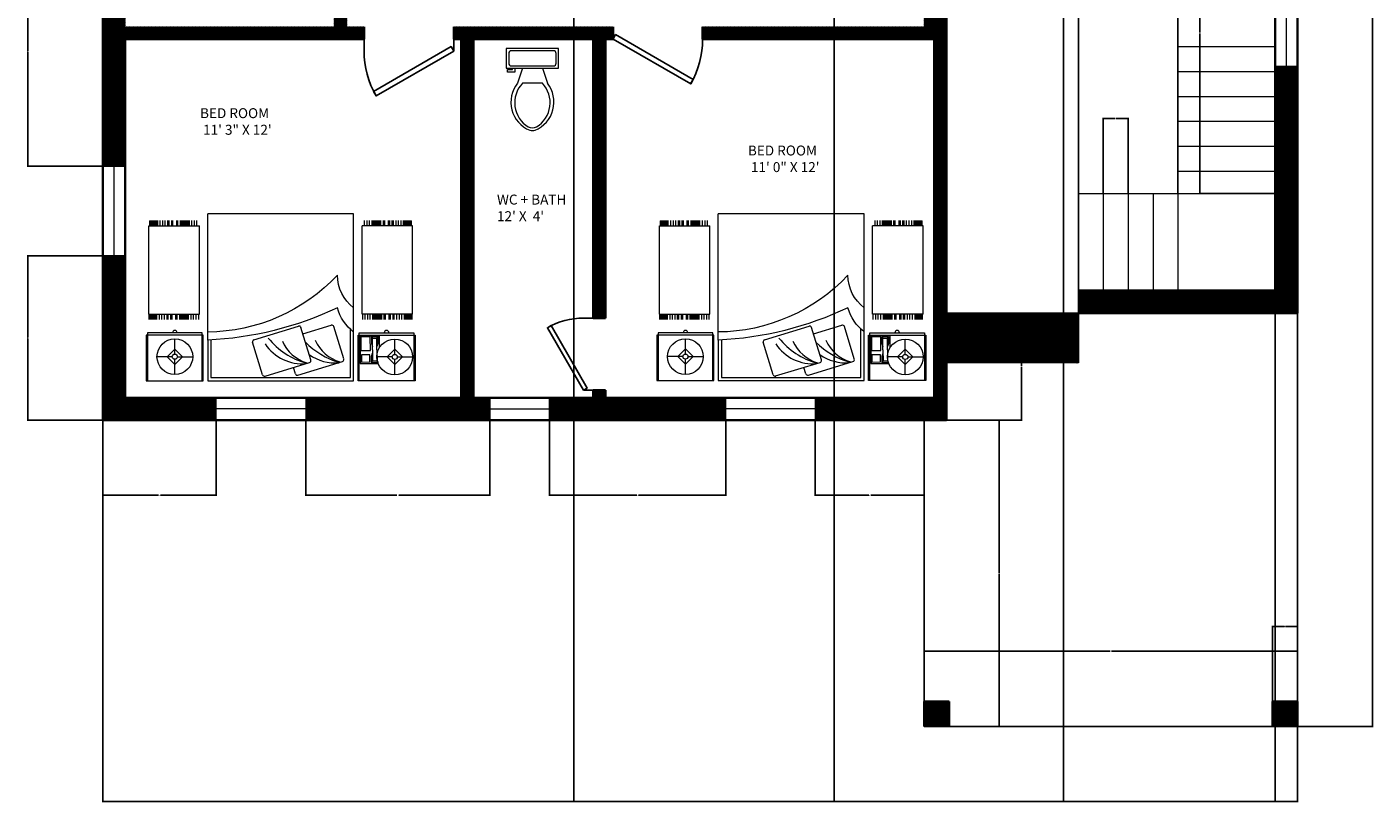
# Model space of a CAD drawing. Units: inches. Extents: x -24 to 516, y -23 to 640.
# Tile 1 of 5: x -24 to 516, y -23 to 288. Entities that reach past the tile are written whole.
import ezdxf

# ---------------------------------------------------------------- set-up
doc = ezdxf.new("R2010")
doc.units = ezdxf.units.IN
doc.header["$MEASUREMENT"] = 0
for name, color, linetype, lineweight in [('A-ANNO-DIMS', 2, 'Continuous', 18), ('A-AREA-IDEN', 7, 'Continuous', 18), ('A-COLS', 7, 'Continuous', 35), ('A-FLOR-STRS', 7, 'Continuous', 18), ('A-SITE-PARK', 8, 'Continuous', 25), ('A-WALL', 7, 'Continuous', 35), ('bathroom', 90, 'Continuous', 18), ('bedroom', 120, 'Continuous', 18), ('doors', 40, 'Continuous', 25), ('window', 30, 'Continuous', 18)]:
    doc.layers.add(name, color=color, linetype=linetype, lineweight=lineweight)
for name, color, linetype, lineweight, true_color in [('A-COLS-PATT', 198, 'Continuous', 13, 0x2e0f2e), ('A-FLOR-STRS-PATT', 51, 'Continuous', 13, 0xf8f6b0), ('A-WALL-PATT', 198, 'Continuous', 13, 0x2e0f2e)]:
    doc.layers.add(name, color=color, linetype=linetype, lineweight=lineweight, true_color=true_color)
doc.styles.get("Standard").update_dxf_attribs({"font": 'arial.ttf'})
doc.dimstyles.get("Standard").update_dxf_attribs({"dimtxt": 0.18, "dimasz": 0.18, "dimexe": 0.18, "dimexo": 0.0625, "dimgap": 0.09, "dimtad": 0, "dimtih": 1, "dimtoh": 1, "dimdec": 4, "dimzin": 0, "dimdsep": 46, "dimtxsty": 'Standard', "dimcen": 0.09, "dimadec": 0, "dimazin": 0, "dimtfac": 1, "dimtdec": 4, "dimtofl": 0, "dimtmove": 0, "dimatfit": 3, "dimfxl": 1, "dimtolj": 1, "dimtzin": 0, "dimarcsym": 0})
pattern_1 = [(45, (-12045.43418, -42625.98622), (-0.08838834765, 0.08838834765), [])]

# ---------------------------------------------------------------- blocks, each defined once
blk = doc.blocks.new('*U10')
for p, q in [((0, 0), (0, 100)), ((750, 0), (750, 100))]:
    blk.add_line(p, q)
blk.add_lwpolyline([(0, 0), (650, -375), (671, -337), (22, 38)], close=True)
blk.add_arc((0, 0), 750, 330, 0)
blk = doc.blocks.new('*U6')
for p, q in [((0, 0), (0, -100)), ((750, 0), (750, -100))]:
    blk.add_line(p, q)
blk.add_lwpolyline([(0, 0), (650, 375), (671, 337), (22, -38)], close=True)
blk.add_arc((0, 0), 750, 0, 30)
blk = doc.blocks.new('3')
for p, q in [((185.866, 224.677), (185.866, 225.236)), ((185.866, 225.236), (186.566, 225.236)), ((185.88, 224.649), (185.88, 225.236)), ((186.116, 225.164), (186.116, 224.976)), ((186.552, 225.236), (186.552, 224.649)), ((186.566, 225.236), (186.566, 224.677)), ((186.62, 225.236), (186.62, 224.64)), ((188.409, 225.236), (186.62, 225.236)), ((187.303, 225.168), (186.758, 225.001)), ((187.706, 225.179), (187.161, 225.012)), ((187.334, 225.152), (187.359, 225.073)), ((187.737, 225.163), (187.858, 224.766)), ((188.409, 224.739), (188.409, 225.236)), ((188.463, 225.236), (188.463, 224.677)), ((189.162, 225.236), (188.463, 225.236)), ((188.477, 225.236), (188.477, 224.649)), ((188.812, 225.162), (188.812, 224.974)), ((189.148, 224.649), (189.148, 225.236)), ((189.162, 224.677), (189.162, 225.236)), ((186.022, 224.945), (186.116, 225.039)), ((186.116, 225.039), (186.21, 224.945)), ((186.54, 225.027), (186.319, 225.027)), ((186.321, 225.017), (186.401, 225.017)), ((186.333, 224.997), (186.321, 225.017)), ((186.334, 224.858), (186.333, 224.997)), ((186.333, 224.997), (186.389, 224.997)), ((186.401, 225.017), (186.389, 224.997)), ((186.39, 224.858), (186.389, 224.997)), ((186.401, 225.017), (186.401, 224.938)), ((186.541, 224.69), (186.54, 225.027)), ((187.144, 224.981), (187.266, 224.584)), ((188.812, 225.036), (188.718, 224.942)), ((188.907, 224.942), (188.812, 225.036)), ((186.084, 224.945), (185.896, 224.945)), ((186.116, 224.851), (186.022, 224.945)), ((186.21, 224.945), (186.116, 224.851)), ((186.116, 224.914), (186.116, 224.726)), ((186.147, 224.945), (186.335, 224.945)), ((186.302, 224.83), (186.303, 224.689)), ((186.322, 224.779), (186.334, 224.818)), ((186.331, 224.905), (186.334, 224.898)), ((186.334, 224.858), (186.334, 224.719)), ((186.401, 224.938), (186.389, 224.898)), ((186.39, 224.858), (186.39, 224.719)), ((186.402, 224.779), (186.39, 224.819)), ((186.742, 224.97), (186.863, 224.573)), ((188.781, 224.942), (188.593, 224.942)), ((188.718, 224.942), (188.812, 224.848)), ((188.812, 224.848), (188.907, 224.942)), ((188.812, 224.911), (188.812, 224.723)), ((188.844, 224.942), (189.032, 224.942)), ((186.566, 224.677), (185.866, 224.677)), ((186.552, 224.649), (185.88, 224.649)), ((186.303, 224.689), (186.541, 224.69)), ((186.323, 224.699), (186.322, 224.779)), ((186.334, 224.719), (186.323, 224.699)), ((186.323, 224.699), (186.402, 224.7)), ((186.334, 224.719), (186.39, 224.719)), ((186.402, 224.7), (186.39, 224.719)), ((186.402, 224.7), (186.402, 224.779)), ((187.242, 224.663), (186.894, 224.557)), ((187.842, 224.735), (187.297, 224.568)), ((188.409, 224.739), (188.409, 223.191)), ((188.463, 224.677), (189.162, 224.677)), ((188.477, 224.649), (189.148, 224.649)), ((185.904, 224.485, -0.909), (185.904, 224.42, -0.909)), ((185.92, 224.485, -0.909), (185.92, 224.42, -0.909)), ((185.92, 224.485, -0.909), (185.92, 224.42, -0.909)), ((185.935, 224.485, -0.909), (185.935, 224.42, -0.909)), ((185.951, 224.485, -0.909), (185.951, 224.42, -0.909)), ((185.966, 224.485, -0.909), (185.966, 224.42, -0.909)), ((185.982, 224.485, -0.909), (185.982, 224.42, -0.909)), ((185.997, 224.485, -0.909), (185.997, 224.42, -0.909)), ((186.028, 224.485, -0.909), (186.028, 224.42, -0.909)), ((186.059, 224.485, -0.909), (186.059, 224.42, -0.909)), ((186.09, 224.485, -0.909), (186.09, 224.42, -0.909)), ((186.09, 224.485, -0.909), (186.09, 224.42, -0.909)), ((186.121, 224.485, -0.909), (186.121, 224.42, -0.909)), ((186.137, 224.485, -0.909), (186.137, 224.42, -0.909)), ((186.168, 224.485, -0.909), (186.168, 224.42, -0.909)), ((186.183, 224.485, -0.909), (186.183, 224.42, -0.909)), ((186.23, 224.485, -0.909), (186.23, 224.42, -0.909)), ((186.245, 224.485, -0.909), (186.245, 224.42, -0.909)), ((186.276, 224.485, -0.909), (186.276, 224.42, -0.909)), ((186.292, 224.485, -0.909), (186.292, 224.42, -0.909)), ((186.307, 224.485, -0.909), (186.307, 224.42, -0.909)), ((186.323, 224.485, -0.909), (186.323, 224.42, -0.909)), ((186.338, 224.485, -0.909), (186.338, 224.42, -0.909)), ((186.354, 224.485, -0.909), (186.354, 224.42, -0.909)), ((186.369, 224.485, -0.909), (186.369, 224.42, -0.909)), ((186.385, 224.485, -0.909), (186.385, 224.42, -0.909)), ((186.416, 224.485, -0.909), (186.416, 224.42, -0.909)), ((186.447, 224.485, -0.909), (186.447, 224.42, -0.909)), ((186.478, 224.485, -0.909), (186.478, 224.42, -0.909)), ((186.509, 224.485, -0.909), (186.509, 224.42, -0.909)), ((186.62, 224.64), (186.62, 223.191)), ((188.52, 224.485, -0.909), (188.52, 224.42, -0.909)), ((188.551, 224.485, -0.909), (188.551, 224.42, -0.909)), ((188.582, 224.485, -0.909), (188.582, 224.42, -0.909)), ((188.613, 224.485, -0.909), (188.613, 224.42, -0.909)), ((188.644, 224.485, -0.909), (188.644, 224.42, -0.909)), ((188.66, 224.485, -0.909), (188.66, 224.42, -0.909)), ((188.675, 224.485, -0.909), (188.675, 224.42, -0.909)), ((188.691, 224.485, -0.909), (188.691, 224.42, -0.909)), ((188.706, 224.485, -0.909), (188.706, 224.42, -0.909)), ((188.722, 224.485, -0.909), (188.722, 224.42, -0.909)), ((188.737, 224.485, -0.909), (188.737, 224.42, -0.909)), ((188.753, 224.485, -0.909), (188.753, 224.42, -0.909)), ((188.784, 224.485, -0.909), (188.784, 224.42, -0.909)), ((188.799, 224.485, -0.909), (188.799, 224.42, -0.909)), ((188.846, 224.485, -0.909), (188.846, 224.42, -0.909)), ((188.861, 224.485, -0.909), (188.861, 224.42, -0.909)), ((188.892, 224.485, -0.909), (188.892, 224.42, -0.909)), ((188.908, 224.485, -0.909), (188.908, 224.42, -0.909)), ((188.939, 224.485, -0.909), (188.939, 224.42, -0.909)), ((188.939, 224.485, -0.909), (188.939, 224.42, -0.909)), ((188.97, 224.485, -0.909), (188.97, 224.42, -0.909)), ((189.001, 224.485, -0.909), (189.001, 224.42, -0.909)), ((189.032, 224.485, -0.909), (189.032, 224.42, -0.909)), ((189.047, 224.485, -0.909), (189.047, 224.42, -0.909)), ((189.063, 224.485, -0.909), (189.063, 224.42, -0.909)), ((189.078, 224.485, -0.909), (189.078, 224.42, -0.909)), ((189.094, 224.485, -0.909), (189.094, 224.42, -0.909)), ((189.109, 224.485, -0.909), (189.109, 224.42, -0.909)), ((189.109, 224.485, -0.909), (189.109, 224.42, -0.909)), ((189.125, 224.485, -0.909), (189.125, 224.42, -0.909)), ((185.897, 224.42, -0.909), (185.897, 223.338, -0.909)), ((185.897, 224.42, -0.909), (186.517, 224.42, -0.909)), ((186.517, 224.42, -0.909), (186.517, 223.338, -0.909)), ((189.131, 224.42, -0.909), (188.511, 224.42, -0.909)), ((188.511, 224.42, -0.909), (188.511, 223.338, -0.909)), ((189.131, 224.42, -0.909), (189.131, 223.338, -0.909)), ((185.897, 223.338, -0.909), (186.517, 223.338, -0.909)), ((185.911, 223.338, -0.909), (185.911, 223.279, -0.909)), ((185.911, 223.338, -0.909), (185.911, 223.279, -0.909)), ((185.911, 223.338, -0.909), (185.911, 223.279, -0.909)), ((185.914, 223.338, -0.909), (185.914, 223.273, -0.909)), ((185.929, 223.338, -0.909), (185.929, 223.273, -0.909)), ((185.929, 223.338, -0.909), (185.929, 223.273, -0.909)), ((185.945, 223.338, -0.909), (185.945, 223.273, -0.909)), ((185.96, 223.338, -0.909), (185.96, 223.273, -0.909)), ((185.976, 223.338, -0.909), (185.976, 223.273, -0.909)), ((185.991, 223.338, -0.909), (185.991, 223.273, -0.909)), ((186.007, 223.338, -0.909), (186.007, 223.273, -0.909)), ((186.038, 223.338, -0.909), (186.038, 223.273, -0.909)), ((186.069, 223.338, -0.909), (186.069, 223.273, -0.909)), ((186.1, 223.338, -0.909), (186.1, 223.273, -0.909)), ((186.1, 223.338, -0.909), (186.1, 223.273, -0.909)), ((186.131, 223.338, -0.909), (186.131, 223.273, -0.909)), ((186.146, 223.338, -0.909), (186.146, 223.273, -0.909)), ((186.177, 223.338, -0.909), (186.177, 223.273, -0.909)), ((186.193, 223.338, -0.909), (186.193, 223.273, -0.909)), ((186.239, 223.338, -0.909), (186.239, 223.273, -0.909)), ((186.255, 223.338, -0.909), (186.255, 223.273, -0.909)), ((186.286, 223.338, -0.909), (186.286, 223.273, -0.909)), ((186.301, 223.338, -0.909), (186.301, 223.273, -0.909)), ((186.317, 223.338, -0.909), (186.317, 223.273, -0.909)), ((186.332, 223.338, -0.909), (186.332, 223.273, -0.909)), ((186.348, 223.338, -0.909), (186.348, 223.273, -0.909)), ((186.363, 223.338, -0.909), (186.363, 223.273, -0.909)), ((186.379, 223.338, -0.909), (186.379, 223.273, -0.909)), ((186.394, 223.338, -0.909), (186.394, 223.273, -0.909)), ((186.425, 223.338, -0.909), (186.425, 223.273, -0.909)), ((186.456, 223.338, -0.909), (186.456, 223.273, -0.909)), ((186.487, 223.338, -0.909), (186.487, 223.273, -0.909)), ((189.131, 223.338, -0.909), (188.511, 223.338, -0.909)), ((188.541, 223.338, -0.909), (188.541, 223.273, -0.909)), ((188.572, 223.338, -0.909), (188.572, 223.273, -0.909)), ((188.603, 223.338, -0.909), (188.603, 223.273, -0.909)), ((188.634, 223.338, -0.909), (188.634, 223.273, -0.909)), ((188.65, 223.338, -0.909), (188.65, 223.273, -0.909)), ((188.665, 223.338, -0.909), (188.665, 223.273, -0.909)), ((188.681, 223.338, -0.909), (188.681, 223.273, -0.909)), ((188.696, 223.338, -0.909), (188.696, 223.273, -0.909)), ((188.712, 223.338, -0.909), (188.712, 223.273, -0.909)), ((188.727, 223.338, -0.909), (188.727, 223.273, -0.909)), ((188.743, 223.338, -0.909), (188.743, 223.273, -0.909)), ((188.774, 223.338, -0.909), (188.774, 223.273, -0.909)), ((188.789, 223.338, -0.909), (188.789, 223.273, -0.909)), ((188.836, 223.338, -0.909), (188.836, 223.273, -0.909)), ((188.851, 223.338, -0.909), (188.851, 223.273, -0.909)), ((188.882, 223.338, -0.909), (188.882, 223.273, -0.909)), ((188.898, 223.338, -0.909), (188.898, 223.273, -0.909)), ((188.929, 223.338, -0.909), (188.929, 223.273, -0.909)), ((188.929, 223.338, -0.909), (188.929, 223.273, -0.909)), ((188.96, 223.338, -0.909), (188.96, 223.273, -0.909)), ((188.991, 223.338, -0.909), (188.991, 223.273, -0.909)), ((189.022, 223.338, -0.909), (189.022, 223.273, -0.909)), ((189.037, 223.338, -0.909), (189.037, 223.273, -0.909)), ((189.053, 223.338, -0.909), (189.053, 223.273, -0.909)), ((189.068, 223.338, -0.909), (189.068, 223.273, -0.909)), ((189.084, 223.338, -0.909), (189.084, 223.273, -0.909)), ((189.099, 223.338, -0.909), (189.099, 223.273, -0.909)), ((189.099, 223.338, -0.909), (189.099, 223.273, -0.909)), ((189.115, 223.338, -0.909), (189.115, 223.273, -0.909)), ((189.117, 223.338, -0.909), (189.117, 223.279, -0.909)), ((189.117, 223.338, -0.909), (189.117, 223.279, -0.909)), ((189.117, 223.338, -0.909), (189.117, 223.279, -0.909)), ((186.62, 223.191), (188.409, 223.191))]:
    blk.add_line(p, q)
blk.add_lwpolyline([(188.369, 224.737), (188.369, 225.197), (186.66, 225.197), (186.66, 224.606)])
for points in [[(186.422, 225.007), (186.422, 224.92), (186.525, 224.92), (186.525, 225.008)], [(186.415, 224.866), (186.416, 224.7), (186.531, 224.7), (186.53, 224.867)]]:
    blk.add_lwpolyline(points, close=True)
for points in [[(186.62, 224.64, -0.162278), (186.819, 224.342, -0.100664), (188.409, 224.739, -0.100664)], [(186.62, 224.342, -0.236068), (186.819, 223.944, -0.205258), (188.409, 224.64, -0.205258)]]:
    blk.add_lwpolyline(points, format="xyb")
for centre, radius in [((186.116, 224.945), 0.219), ((188.812, 224.942), 0.219), ((186.116, 224.945), 0.0313), ((188.812, 224.942), 0.0313)]:
    blk.add_circle(centre, radius)
for centre, radius, start, end in [((187.311, 225.145), 0.0248, 17.0142, 107.0142), ((187.713, 225.156), 0.0248, 17.0142, 107.0142), ((186.765, 224.978), 0.0248, 107.0142, 197.0142), ((186.647, 224.541), 0.487, 24.2209, 73.0691), ((186.848, 224.471), 0.547, 54.6851, 95.1605), ((186.536, 224.105), 0.943, 44.2727, 73.7189), ((187.168, 224.989), 0.0248, 107.0142, 197.0142), ((187.05, 224.552), 0.487, 24.2209, 73.0691), ((187.25, 224.482), 0.547, 33.7801, 95.1605), ((186.938, 224.116), 0.943, 39.4023, 73.7189), ((186.216, 224.649), 0.028, 180, 0), ((187.835, 224.758), 0.0248, 287.0142, 17.0142), ((188.812, 224.649), 0.028, 180, 0), ((186.887, 224.581), 0.0248, 197.0142, 287.0142), ((187.289, 224.592), 0.0248, 197.0142, 287.0142)]:
    blk.add_arc(centre, radius, start, end)
blk = doc.blocks.new('Toilet - top')
for p, q in [((9.5, -6), (9.5, -2)), ((-10, -8.5), (-8, -8.5)), ((-10, -9.5), (-10, -8.5)), ((-7, -9.5), (-10, -9.5)), ((-8, -8.5), (-8, -8)), ((-7, -8), (-7, -9.5)), ((-4, -8), (-6, -14)), ((4, -8), (6, -14)), ((4, -14), (-4, -14))]:
    blk.add_line(p, q)
blk.add_lwpolyline([(10.5, -8), (10.5, 0), (-10.5, 0), (-10.5, -8)], close=True)
for points in [[(-9.5, -2), (-9.5, -6)], [(8.5, -1), (-8.5, -1)], [(-8.5, -7), (8.5, -7)]]:
    blk.add_lwpolyline(points)
for centre, radius, start, end in [((-8.62, -1.88), 0.884, 81.8699, 188.1301), ((8.62, -1.88), 0.884, 351.8699, 98.1301), ((-8.62, -6.12), 0.884, 171.8699, 278.1301), ((8.62, -6.12), 0.884, 261.8699, 8.1301), ((3.52, -21.58), 12.17, 141.4691, 247.9714), ((4.2, -21.82), 11.33, 136.3677, 238.9468), ((-3.52, -21.58), 12.17, 292.0284, 38.5307), ((-4.2, -21.82), 11.33, 301.053, 43.6321), ((0, -27.88), 4, 245.7318, 294.2682), ((0, -29), 4, 254.8605, 285.1395)]:
    blk.add_arc(centre, radius, start, end)
blk = doc.blocks.new('WIN-36IN')
for p, q in [((0, 0), (0, 36)), ((0, 36), (9, 36)), ((4.5, 0), (4.5, 36)), ((9, 36), (9, 0)), ((9, 0), (0, 0)), ((9, 0), (4.5, 0))]:
    blk.add_line(p, q)
blk = doc.blocks.new('WIN-24IN')
for p, q in [((0, 0), (0, 24)), ((0, 24), (9, 24)), ((4.5, 0), (4.5, 24)), ((9, 24), (9, 0)), ((9, 0), (0, 0)), ((9, 0), (4.5, 0))]:
    blk.add_line(p, q)
blk = doc.blocks.new('WIN-48IN')
for p, q in [((0, 48), (9, 48)), ((0, 0), (0, 48)), ((4.5, 48), (4.5, 0)), ((9, 48), (9, 0)), ((9, 0), (0, 0))]:
    blk.add_line(p, q)
blk = doc.blocks.new('*D33')
at = {"layer": 'A-ANNO-DIMS', "color": 0, "lineweight": -2, "transparency": 16777216}
for p, q in [((6.09, 129.95), (6.09, -23.35)), ((486.09, 6.95), (486.09, -23.35)), ((6.27, -23.17), (245.8, -23.17)), ((485.91, -23.17), (246.38, -23.17))]:
    blk.add_line(p, q, dxfattribs=at)
at = {"layer": 'A-ANNO-DIMS', "color": 0, "transparency": 16777216}
for points in [[(6.27, -23.14), (6.27, -23.2), (6.09, -23.17)], [(485.91, -23.14), (485.91, -23.2), (486.09, -23.17)]]:
    blk.add_solid(points, dxfattribs=at)
at = {"layer": 'Defpoints', "color": 0, "transparency": 16777216}
for p in [(6.09, 130.01), (486.09, 7.01), (486.09, -23.17)]:
    blk.add_point(p, dxfattribs=at)
at = {"layer": 'A-ANNO-DIMS', "color": 0, "transparency": 16777216, "insert": (246.09, -23.17), "char_height": 0.18, "attachment_point": 5}
blk.add_mtext('\\A1;480', dxfattribs=at)
blk = doc.blocks.new('*D34')
at = {"layer": 'A-ANNO-DIMS', "color": 0, "lineweight": -2, "transparency": 16777216}
for p, q in [((486.15, 610.01), (516.45, 610.01)), ((516.27, 609.83), (516.27, 308.7)), ((516.27, 7.19), (516.27, 308.33)), ((486.15, 7.01), (516.45, 7.01))]:
    blk.add_line(p, q, dxfattribs=at)
at = {"layer": 'A-ANNO-DIMS', "color": 0, "transparency": 16777216}
for points in [[(516.24, 609.83), (516.3, 609.83), (516.27, 610.01)], [(516.24, 7.19), (516.3, 7.19), (516.27, 7.01)]]:
    blk.add_solid(points, dxfattribs=at)
at = {"layer": 'Defpoints', "color": 0, "transparency": 16777216}
for p in [(486.09, 610.01), (516.27, 610.01), (486.09, 7.01)]:
    blk.add_point(p, dxfattribs=at)
at = {"layer": 'A-ANNO-DIMS', "color": 0, "transparency": 16777216, "insert": (516.27, 308.51), "char_height": 0.18, "attachment_point": 5}
blk.add_mtext('\\A1;603', dxfattribs=at)
blk = doc.blocks.new('*D35')
at = {"layer": 'A-ANNO-DIMS', "color": 0, "lineweight": -2, "transparency": 16777216}
for p, q in [((336.15, 130.01), (366.45, 130.01)), ((366.27, 129.83), (366.27, 68.7)), ((366.27, 7.19), (366.27, 68.33)), ((336.15, 7.01), (366.45, 7.01))]:
    blk.add_line(p, q, dxfattribs=at)
at = {"layer": 'A-ANNO-DIMS', "color": 0, "transparency": 16777216}
for points in [[(366.24, 129.83), (366.3, 129.83), (366.27, 130.01)], [(366.24, 7.19), (366.3, 7.19), (366.27, 7.01)]]:
    blk.add_solid(points, dxfattribs=at)
at = {"layer": 'Defpoints', "color": 0, "transparency": 16777216}
for p in [(336.09, 130.01), (336.09, 7.01), (366.27, 7.01)]:
    blk.add_point(p, dxfattribs=at)
at = {"layer": 'A-ANNO-DIMS', "color": 0, "transparency": 16777216, "insert": (366.27, 68.51), "char_height": 0.18, "attachment_point": 5}
blk.add_mtext('\\A1;123', dxfattribs=at)
blk = doc.blocks.new('*D36')
at = {"layer": 'A-ANNO-DIMS', "color": 0, "lineweight": -2, "transparency": 16777216}
for p, q in [((6.09, 129.95), (6.09, 99.65)), ((51.66, 129.95), (51.66, 99.65)), ((6.27, 99.83), (28.48, 99.83)), ((51.48, 99.83), (29.27, 99.83))]:
    blk.add_line(p, q, dxfattribs=at)
at = {"layer": 'A-ANNO-DIMS', "color": 0, "transparency": 16777216}
for points in [[(6.27, 99.86), (6.27, 99.8), (6.09, 99.83)], [(51.48, 99.86), (51.48, 99.8), (51.66, 99.83)]]:
    blk.add_solid(points, dxfattribs=at)
at = {"layer": 'Defpoints', "color": 0, "transparency": 16777216}
for p in [(6.09, 130.01), (51.66, 130.01), (6.09, 99.83)]:
    blk.add_point(p, dxfattribs=at)
at = {"layer": 'A-ANNO-DIMS', "color": 0, "transparency": 16777216, "insert": (28.88, 99.83), "char_height": 0.18, "attachment_point": 5}
blk.add_mtext('\\A1;45.58', dxfattribs=at)
blk = doc.blocks.new('*D37')
at = {"layer": 'A-ANNO-DIMS', "color": 0, "lineweight": -2, "transparency": 16777216}
for p, q in [((87.66, 129.95), (87.66, 99.65)), ((161.63, 129.95), (161.63, 99.65)), ((87.84, 99.83), (124.25, 99.83)), ((161.45, 99.83), (125.04, 99.83))]:
    blk.add_line(p, q, dxfattribs=at)
at = {"layer": 'A-ANNO-DIMS', "color": 0, "transparency": 16777216}
for points in [[(87.84, 99.86), (87.84, 99.8), (87.66, 99.83)], [(161.45, 99.86), (161.45, 99.8), (161.63, 99.83)]]:
    blk.add_solid(points, dxfattribs=at)
at = {"layer": 'Defpoints', "color": 0, "transparency": 16777216}
for p in [(87.66, 130.01), (161.63, 130.01), (87.66, 99.83)]:
    blk.add_point(p, dxfattribs=at)
at = {"layer": 'A-ANNO-DIMS', "color": 0, "transparency": 16777216, "insert": (124.65, 99.83), "char_height": 0.18, "attachment_point": 5}
blk.add_mtext('\\A1;73.97', dxfattribs=at)
blk = doc.blocks.new('*D38')
at = {"layer": 'A-ANNO-DIMS', "color": 0, "lineweight": -2, "transparency": 16777216}
for p, q in [((185.63, 129.95), (185.63, 99.65)), ((256.35, 129.95), (256.35, 99.65)), ((185.81, 99.83), (220.6, 99.83)), ((256.17, 99.83), (221.38, 99.83))]:
    blk.add_line(p, q, dxfattribs=at)
at = {"layer": 'A-ANNO-DIMS', "color": 0, "transparency": 16777216}
for points in [[(185.81, 99.86), (185.81, 99.8), (185.63, 99.83)], [(256.17, 99.86), (256.17, 99.8), (256.35, 99.83)]]:
    blk.add_solid(points, dxfattribs=at)
at = {"layer": 'Defpoints', "color": 0, "transparency": 16777216}
for p in [(185.63, 130.01), (256.35, 130.01), (185.63, 99.83)]:
    blk.add_point(p, dxfattribs=at)
at = {"layer": 'A-ANNO-DIMS', "color": 0, "transparency": 16777216, "insert": (220.99, 99.83), "char_height": 0.18, "attachment_point": 5}
blk.add_mtext('\\A1;70.72', dxfattribs=at)
blk = doc.blocks.new('*D39')
at = {"layer": 'A-ANNO-DIMS', "color": 0, "lineweight": -2, "transparency": 16777216}
for p, q in [((292.35, 129.95), (292.35, 99.65)), ((336.09, 129.95), (336.09, 99.65)), ((292.53, 99.83), (313.82, 99.83)), ((335.91, 99.83), (314.62, 99.83))]:
    blk.add_line(p, q, dxfattribs=at)
at = {"layer": 'A-ANNO-DIMS', "color": 0, "transparency": 16777216}
for points in [[(292.53, 99.86), (292.53, 99.8), (292.35, 99.83)], [(335.91, 99.86), (335.91, 99.8), (336.09, 99.83)]]:
    blk.add_solid(points, dxfattribs=at)
at = {"layer": 'Defpoints', "color": 0, "transparency": 16777216}
for p in [(292.35, 130.01), (336.09, 130.01), (292.35, 99.83)]:
    blk.add_point(p, dxfattribs=at)
at = {"layer": 'A-ANNO-DIMS', "color": 0, "transparency": 16777216, "insert": (314.22, 99.83), "char_height": 0.18, "attachment_point": 5}
blk.add_mtext('\\A1;43.74', dxfattribs=at)
blk = doc.blocks.new('*D40')
at = {"layer": 'A-ANNO-DIMS', "color": 0, "lineweight": -2, "transparency": 16777216}
for p, q in [((336.09, 7.08), (336.09, 37.38)), ((336.27, 37.2), (410.81, 37.2)), ((485.91, 37.2), (411.37, 37.2)), ((486.09, 7.08), (486.09, 37.38))]:
    blk.add_line(p, q, dxfattribs=at)
at = {"layer": 'A-ANNO-DIMS', "color": 0, "transparency": 16777216}
for points in [[(336.27, 37.23), (336.27, 37.17), (336.09, 37.2)], [(485.91, 37.23), (485.91, 37.17), (486.09, 37.2)]]:
    blk.add_solid(points, dxfattribs=at)
at = {"layer": 'Defpoints', "color": 0, "transparency": 16777216}
for p in [(486.09, 37.2), (336.09, 7.01), (486.09, 7.01)]:
    blk.add_point(p, dxfattribs=at)
at = {"layer": 'A-ANNO-DIMS', "color": 0, "transparency": 16777216, "insert": (411.09, 37.2), "char_height": 0.18, "attachment_point": 5}
blk.add_mtext('\\A1;150', dxfattribs=at)
blk = doc.blocks.new('*D41')
at = {"layer": 'A-ANNO-DIMS', "color": 0, "lineweight": -2, "transparency": 16777216}
for p, q in [((6.03, 195.95), (-24.28, 195.95)), ((-24.1, 195.77), (-24.1, 163.16)), ((-24.1, 130.19), (-24.1, 162.8)), ((6.03, 130.01), (-24.28, 130.01))]:
    blk.add_line(p, q, dxfattribs=at)
at = {"layer": 'A-ANNO-DIMS', "color": 0, "transparency": 16777216}
for points in [[(-24.13, 195.77), (-24.07, 195.77), (-24.1, 195.95)], [(-24.13, 130.19), (-24.07, 130.19), (-24.1, 130.01)]]:
    blk.add_solid(points, dxfattribs=at)
at = {"layer": 'Defpoints', "color": 0, "transparency": 16777216}
for p in [(-24.1, 195.95), (6.09, 195.95), (6.09, 130.01)]:
    blk.add_point(p, dxfattribs=at)
at = {"layer": 'A-ANNO-DIMS', "color": 0, "transparency": 16777216, "insert": (-24.1, 162.98), "char_height": 0.18, "attachment_point": 5}
blk.add_mtext('\\A1;65.93', dxfattribs=at)
blk = doc.blocks.new('*D42')
at = {"layer": 'A-ANNO-DIMS', "color": 0, "lineweight": -2, "transparency": 16777216}
for p, q in [((6.03, 324.05), (-24.28, 324.05)), ((-24.1, 323.87), (-24.1, 278.18)), ((-24.1, 232.13), (-24.1, 277.81)), ((6.03, 231.95), (-24.28, 231.95))]:
    blk.add_line(p, q, dxfattribs=at)
at = {"layer": 'A-ANNO-DIMS', "color": 0, "transparency": 16777216}
for points in [[(-24.13, 323.87), (-24.07, 323.87), (-24.1, 324.05)], [(-24.13, 232.13), (-24.07, 232.13), (-24.1, 231.95)]]:
    blk.add_solid(points, dxfattribs=at)
at = {"layer": 'Defpoints', "color": 0, "transparency": 16777216}
for p in [(-24.1, 324.05), (6.09, 324.05), (6.09, 231.95)]:
    blk.add_point(p, dxfattribs=at)
at = {"layer": 'A-ANNO-DIMS', "color": 0, "transparency": 16777216, "insert": (-24.1, 278), "char_height": 0.18, "attachment_point": 5}
blk.add_mtext('\\A1;92.1', dxfattribs=at)
blk = doc.blocks.new('*D49')
at = {"layer": 'A-ANNO-DIMS', "color": 0, "lineweight": -2, "transparency": 16777216}
for p, q in [((345.09, 173.08), (345.09, 640.38)), ((345.27, 640.2), (371.37, 640.2)), ((397.91, 640.2), (371.81, 640.2)), ((398.09, 173.08), (398.09, 640.38))]:
    blk.add_line(p, q, dxfattribs=at)
at = {"layer": 'A-ANNO-DIMS', "color": 0, "transparency": 16777216}
for points in [[(345.27, 640.23), (345.27, 640.17), (345.09, 640.2)], [(397.91, 640.23), (397.91, 640.17), (398.09, 640.2)]]:
    blk.add_solid(points, dxfattribs=at)
at = {"layer": 'Defpoints', "color": 0, "transparency": 16777216}
for p in [(398.09, 640.2), (345.09, 173.01), (398.09, 173.01)]:
    blk.add_point(p, dxfattribs=at)
at = {"layer": 'A-ANNO-DIMS', "color": 0, "transparency": 16777216, "insert": (371.59, 640.2), "char_height": 0.18, "attachment_point": 5}
blk.add_mtext('\\A1;53', dxfattribs=at)
blk = doc.blocks.new('*D51')
at = {"layer": 'A-ANNO-DIMS', "color": 0, "lineweight": -2, "transparency": 16777216}
for p, q in [((438.09, 221.08), (438.09, 640.38)), ((438.27, 640.2), (457.37, 640.2)), ((476.91, 640.2), (457.81, 640.2)), ((477.09, 221.08), (477.09, 640.38))]:
    blk.add_line(p, q, dxfattribs=at)
at = {"layer": 'A-ANNO-DIMS', "color": 0, "transparency": 16777216}
for points in [[(438.27, 640.23), (438.27, 640.17), (438.09, 640.2)], [(476.91, 640.23), (476.91, 640.17), (477.09, 640.2)]]:
    blk.add_solid(points, dxfattribs=at)
at = {"layer": 'Defpoints', "color": 0, "transparency": 16777216}
for p in [(477.09, 640.2), (438.09, 221.01), (477.09, 221.01)]:
    blk.add_point(p, dxfattribs=at)
at = {"layer": 'A-ANNO-DIMS', "color": 0, "transparency": 16777216, "insert": (457.59, 640.2), "char_height": 0.18, "attachment_point": 5}
blk.add_mtext('\\A1;39', dxfattribs=at)
blk = doc.blocks.new('*D54')
at = {"layer": 'A-ANNO-DIMS', "color": 0, "lineweight": -2, "transparency": 16777216}
for p, q in [((392.09, 397.95), (392.09, -23.35)), ((477.09, 397.95), (477.09, -23.35)), ((392.27, -23.17), (434.37, -23.17)), ((476.91, -23.17), (434.81, -23.17))]:
    blk.add_line(p, q, dxfattribs=at)
at = {"layer": 'A-ANNO-DIMS', "color": 0, "transparency": 16777216}
for points in [[(392.27, -23.14), (392.27, -23.2), (392.09, -23.17)], [(476.91, -23.14), (476.91, -23.2), (477.09, -23.17)]]:
    blk.add_solid(points, dxfattribs=at)
at = {"layer": 'Defpoints', "color": 0, "transparency": 16777216}
for p in [(392.09, 398.01), (477.09, 398.01), (477.09, -23.17)]:
    blk.add_point(p, dxfattribs=at)
at = {"layer": 'A-ANNO-DIMS', "color": 0, "transparency": 16777216, "insert": (434.59, -23.17), "char_height": 0.18, "attachment_point": 5}
blk.add_mtext('\\A1;85', dxfattribs=at)
blk = doc.blocks.new('*D55')
at = {"layer": 'A-ANNO-DIMS', "color": 0, "lineweight": -2, "transparency": 16777216}
for p, q in [((195.37, 401.52), (195.37, -23.35)), ((299.94, 401.52), (299.94, -23.35)), ((195.55, -23.17), (247.2, -23.17)), ((299.76, -23.17), (248.11, -23.17))]:
    blk.add_line(p, q, dxfattribs=at)
at = {"layer": 'A-ANNO-DIMS', "color": 0, "transparency": 16777216}
for points in [[(195.55, -23.14), (195.55, -23.2), (195.37, -23.17)], [(299.76, -23.14), (299.76, -23.2), (299.94, -23.17)]]:
    blk.add_solid(points, dxfattribs=at)
at = {"layer": 'Defpoints', "color": 0, "transparency": 16777216}
for p in [(195.37, 401.58), (299.94, 401.58), (299.94, -23.17)]:
    blk.add_point(p, dxfattribs=at)
at = {"layer": 'A-ANNO-DIMS', "color": 0, "transparency": 16777216, "insert": (247.66, -23.17), "char_height": 0.18, "attachment_point": 5}
blk.add_mtext('\\A1;104.57', dxfattribs=at)
blk = doc.blocks.new('*D58')
at = {"layer": 'A-ANNO-DIMS', "color": 0, "lineweight": -2, "transparency": 16777216}
for p, q in [((345.15, 173.01), (375.45, 173.01)), ((375.27, 172.83), (375.27, 151.7)), ((375.27, 130.19), (375.27, 151.33)), ((345.15, 130.01), (375.45, 130.01))]:
    blk.add_line(p, q, dxfattribs=at)
at = {"layer": 'A-ANNO-DIMS', "color": 0, "transparency": 16777216}
for points in [[(375.24, 172.83), (375.3, 172.83), (375.27, 173.01)], [(375.24, 130.19), (375.3, 130.19), (375.27, 130.01)]]:
    blk.add_solid(points, dxfattribs=at)
at = {"layer": 'Defpoints', "color": 0, "transparency": 16777216}
for p in [(345.09, 173.01), (345.09, 130.01), (375.27, 130.01)]:
    blk.add_point(p, dxfattribs=at)
at = {"layer": 'A-ANNO-DIMS', "color": 0, "transparency": 16777216, "insert": (375.27, 151.51), "char_height": 0.18, "attachment_point": 5}
blk.add_mtext('\\A1;43', dxfattribs=at)
blk = doc.blocks.new('*D59')
at = {"layer": 'A-ANNO-DIMS', "color": 0, "lineweight": -2, "transparency": 16777216}
for p, q in [((477.03, 350.01), (446.72, 350.01)), ((446.9, 349.83), (446.9, 285.7)), ((446.9, 221.19), (446.9, 285.33)), ((477.03, 221.01), (446.72, 221.01))]:
    blk.add_line(p, q, dxfattribs=at)
at = {"layer": 'A-ANNO-DIMS', "color": 0, "transparency": 16777216}
for points in [[(446.87, 349.83), (446.93, 349.83), (446.9, 350.01)], [(446.87, 221.19), (446.93, 221.19), (446.9, 221.01)]]:
    blk.add_solid(points, dxfattribs=at)
at = {"layer": 'Defpoints', "color": 0, "transparency": 16777216}
for p in [(446.9, 350.01), (477.09, 350.01), (477.09, 221.01)]:
    blk.add_point(p, dxfattribs=at)
at = {"layer": 'A-ANNO-DIMS', "color": 0, "transparency": 16777216, "insert": (446.9, 285.51), "char_height": 0.18, "attachment_point": 5}
blk.add_mtext('\\A1;129', dxfattribs=at)
blk = doc.blocks.new('*D66')
at = {"layer": 'A-ANNO-DIMS', "color": 0, "lineweight": -2, "transparency": 16777216}
for p, q in [((476.09, 17.08), (476.09, 47.38)), ((476.27, 47.2), (480.88, 47.2)), ((485.91, 47.2), (481.3, 47.2)), ((486.09, 17.08), (486.09, 47.38))]:
    blk.add_line(p, q, dxfattribs=at)
at = {"layer": 'A-ANNO-DIMS', "color": 0, "transparency": 16777216}
for points in [[(476.27, 47.23), (476.27, 47.17), (476.09, 47.2)], [(485.91, 47.23), (485.91, 47.17), (486.09, 47.2)]]:
    blk.add_solid(points, dxfattribs=at)
at = {"layer": 'Defpoints', "color": 0, "transparency": 16777216}
for p in [(486.09, 47.2), (476.09, 17.01), (486.09, 17.01)]:
    blk.add_point(p, dxfattribs=at)
at = {"layer": 'A-ANNO-DIMS', "color": 0, "transparency": 16777216, "insert": (481.09, 47.2), "char_height": 0.18, "attachment_point": 5}
blk.add_mtext('\\A1;10', dxfattribs=at)
blk = doc.blocks.new('*D67')
at = {"layer": 'A-ANNO-DIMS', "color": 0, "lineweight": -2, "transparency": 16777216}
for p, q in [((408.09, 221.08), (408.09, 251.38)), ((408.27, 251.2), (412.88, 251.2)), ((417.91, 251.2), (413.3, 251.2)), ((418.09, 221.08), (418.09, 251.38))]:
    blk.add_line(p, q, dxfattribs=at)
at = {"layer": 'A-ANNO-DIMS', "color": 0, "transparency": 16777216}
for points in [[(408.27, 251.23), (408.27, 251.17), (408.09, 251.2)], [(417.91, 251.23), (417.91, 251.17), (418.09, 251.2)]]:
    blk.add_solid(points, dxfattribs=at)
at = {"layer": 'Defpoints', "color": 0, "transparency": 16777216}
for p in [(418.09, 251.2), (408.09, 221.01), (418.09, 221.01)]:
    blk.add_point(p, dxfattribs=at)
at = {"layer": 'A-ANNO-DIMS', "color": 0, "transparency": 16777216, "insert": (413.09, 251.2), "char_height": 0.18, "attachment_point": 5}
blk.add_mtext('\\A1;10', dxfattribs=at)

msp = doc.modelspace()

# ---------------------------------------------------------------- hatches: boundary and pattern name
at = {"layer": 'A-COLS-PATT'}
h = msp.add_hatch(dxfattribs=at)
h.set_pattern_fill('ANSI31', color=256)
h.set_pattern_definition(pattern_1)
h.paths.add_polyline_path([(346.088, 17.013), (336.088, 17.013), (336.088, 7.013), (346.088, 7.013)])
h.paths.add_polyline_path([(486.088, 17.013), (476.088, 17.013), (476.088, 7.013), (486.088, 7.013)])
at = {"layer": 'A-FLOR-STRS-PATT'}
h = msp.add_hatch(dxfattribs=at)
h.set_pattern_fill('ANSI31', color=256)
h.set_pattern_definition(pattern_1)
h.paths.add_polyline_path([(398.088, 163.013), (345.088, 163.013), (345.088, 153.013), (398.088, 153.013)])
h.paths.add_polyline_path([(398.088, 173.013), (345.088, 173.013), (345.088, 163.013), (398.088, 163.013)])
at = {"layer": 'A-WALL-PATT'}
h = msp.add_hatch(dxfattribs=at)
h.set_pattern_fill('ANSI31', color=256)
h.set_pattern_definition(pattern_1)
h.paths.add_polyline_path([(15.088, 601.013), (52.998, 601.013), (52.998, 610.013), (6.088, 610.013), (6.088, 554.753), (15.088, 554.753)])
h.paths.add_polyline_path([(171.065, 610.013), (88.998, 610.013), (88.998, 601.013), (150.088, 601.013), (150.088, 457.013), (147.088, 457.013), (147.088, 452.013), (155.088, 452.013), (155.088, 488.013), (203.088, 488.013), (203.088, 452.013), (301.088, 452.013), (301.088, 457.013), (208.088, 457.013), (208.088, 496.013), (203.088, 496.013), (203.088, 493.013), (155.088, 493.013), (155.088, 601.013), (171.065, 601.013)])
h.paths.add_polyline_path([(264.208, 610.013), (195.065, 610.013), (195.065, 601.013), (203.088, 601.013), (203.088, 525.013), (208.088, 525.013), (208.088, 601.013), (264.208, 601.013)], flags=17)
h.paths.add_polyline_path([(384.556, 610.013), (300.208, 610.013), (300.208, 601.013), (340.088, 601.013), (340.088, 457.013), (337.088, 456.991), (337.088, 452.013), (340.088, 452.013), (348.088, 452.013), (348.088, 457.013), (345.088, 457.013), (345.088, 601.013), (384.556, 601.013)])
h.paths.add_polyline_path([(486.088, 610.013), (420.556, 610.013), (420.556, 601.013), (477.088, 601.013), (477.088, 564.302), (486.088, 564.302)])
h.paths.add_polyline_path([(486.088, 516.302), (477.088, 516.302), (477.088, 457.013), (387.088, 457.013), (387.088, 430.013), (392.088, 430.013), (392.088, 452.013), (477.088, 452.013), (477.088, 442.706), (486.088, 442.706)])
h.paths.add_polyline_path([(486.088, 418.706), (477.088, 418.706), (477.088, 398.013), (392.088, 398.013), (392.088, 401.013), (388.222, 401.013), (387.088, 401.013), (387.088, 398.013), (336.088, 398.013), (336.088, 386.013), (345.088, 386.013), (345.088, 389.013), (477.088, 389.013), (477.088, 320.013), (486.088, 320.013)])
h.paths.add_polyline_path([(486.088, 272.013), (477.088, 272.013), (477.088, 182.013), (398.088, 182.013), (398.088, 173.013), (486.088, 173.013)])
h = msp.add_hatch(dxfattribs=at)
h.set_pattern_fill('ANSI31', color=256)
h.set_pattern_definition(pattern_1)
h.paths.add_polyline_path([(161.63, 139.013), (155.088, 139.013), (155.088, 283.013), (203.088, 283.013), (203.088, 171.013), (208.088, 171.013), (208.088, 283.013), (211.088, 283.013), (211.088, 288.013), (208.088, 288.013), (147.088, 288.013), (147.088, 283.013), (150.088, 283.013), (150.088, 139.013), (87.664, 139.013), (87.664, 134.513), (87.664, 130.013), (161.63, 130.013)])
h.paths.add_polyline_path([(256.352, 139.013), (208.088, 139.013), (208.088, 142.013), (203.088, 142.013), (203.088, 139.013), (185.63, 139.013), (185.63, 130.013), (256.352, 130.013)])
h.paths.add_polyline_path([(345.088, 326.013), (336.088, 326.013), (336.088, 288.013), (247.088, 288.013), (247.088, 283.013), (340.088, 283.013), (340.088, 139.013), (292.352, 139.013), (292.352, 134.513), (292.352, 130.013), (345.088, 130.013)])
h.paths.add_polyline_path([(51.664, 139.013), (15.088, 139.013), (15.088, 195.946), (10.588, 195.946), (6.088, 195.946), (6.088, 130.013), (51.664, 130.013)])
h.paths.add_polyline_path([(15.088, 283.013), (111.088, 283.013), (111.088, 288.013), (104.088, 288.013), (104.088, 354.013), (99.088, 354.013), (99.088, 288.013), (15.088, 288.013), (15.088, 324.046), (10.588, 324.046), (6.088, 324.046), (6.088, 231.946), (15.088, 231.946)])
h.paths.add_polyline_path([(15.088, 398.013), (99.088, 398.013), (99.088, 390.013), (104.088, 390.013), (104.088, 393.013), (104.088, 407.013), (99.088, 407.013), (99.088, 404.013), (15.088, 404.013), (15.088, 416.474), (10.588, 416.474), (6.088, 416.474), (6.088, 360.046), (15.088, 360.046)])
h.paths.add_polyline_path([(15.088, 518.753), (10.588, 518.753), (6.088, 518.753), (6.088, 440.474), (15.088, 440.474), (15.088, 452.013), (99.088, 452.013), (99.088, 436.013), (104.088, 436.013), (104.088, 452.013), (111.088, 452.013), (111.088, 457.013), (15.088, 457.013)])

# ---------------------------------------------------------------- linework, layer by layer
at = {"layer": 'A-COLS'}
for p, q in [((336.088, 7.013), (336.088, 17.013)), ((336.088, 17.013), (346.088, 17.013)), ((346.088, 17.013), (346.088, 7.013)), ((486.088, 17.013), (476.088, 17.013)), ((476.088, 17.013), (476.088, 7.013)), ((486.088, 7.013), (486.088, 17.013))]:
    msp.add_line(p, q, dxfattribs=at)
at = {"layer": 'A-FLOR-STRS'}
for p, q in [((438.088, 389.013), (438.088, 221.013)), ((438.088, 280.013), (477.088, 280.013)), ((438.088, 270.013), (477.088, 270.013)), ((438.088, 260.013), (477.088, 260.013)), ((438.088, 250.013), (477.088, 250.013)), ((438.088, 240.013), (477.088, 240.013)), ((438.088, 230.013), (477.088, 230.013)), ((398.088, 221.013), (477.088, 221.013)), ((398.088, 221.013), (398.088, 173.013)), ((408.088, 221.013), (408.088, 182.013)), ((418.088, 221.013), (418.088, 182.013)), ((428.088, 221.013), (428.088, 182.013)), ((438.088, 221.013), (438.088, 182.013)), ((398.088, 173.013), (345.088, 173.013)), ((398.088, 173.013), (398.088, 153.013)), ((398.088, 163.013), (345.088, 163.013)), ((398.088, 153.013), (345.088, 153.013))]:
    msp.add_line(p, q, dxfattribs=at)
at = {"layer": 'A-SITE-PARK'}
for p, q in [((486.088, 173.013), (486.088, 7.013)), ((336.088, 7.013), (336.088, 130.013)), ((486.088, 7.013), (336.088, 7.013))]:
    msp.add_line(p, q, dxfattribs=at)
at = {"layer": 'A-WALL'}
for p, q in [((477.088, 389.013), (477.088, 182.013)), ((345.088, 130.013), (345.088, 326.013)), ((111.088, 283.013), (111.088, 288.013)), ((147.088, 288.013), (147.088, 283.013)), ((211.088, 288.013), (211.088, 283.013)), ((247.088, 283.013), (247.088, 288.013)), ((15.088, 283.013), (111.088, 283.013)), ((111.088, 283.013), (15.088, 283.013)), ((15.088, 139.013), (15.088, 283.013)), ((147.088, 283.013), (150.088, 283.013)), ((150.088, 283.013), (147.088, 283.013)), ((150.088, 139.013), (150.088, 283.013)), ((203.088, 283.013), (155.088, 283.013)), ((155.088, 139.013), (155.088, 283.013)), ((203.088, 171.013), (203.088, 283.013)), ((211.088, 283.013), (208.088, 283.013)), ((208.088, 171.013), (208.088, 283.013)), ((340.088, 283.013), (247.088, 283.013)), ((340.088, 139.013), (340.088, 283.013)), ((477.088, 182.013), (398.088, 182.013)), ((208.088, 171.013), (203.088, 171.013)), ((486.088, 173.013), (398.088, 173.013)), ((203.088, 139.013), (203.088, 142.013)), ((203.088, 139.013), (203.088, 142.013)), ((203.088, 142.013), (208.088, 142.013)), ((208.088, 139.013), (208.088, 142.013)), ((150.088, 139.013), (15.088, 139.013)), ((203.088, 139.013), (155.088, 139.013)), ((340.088, 139.013), (208.088, 139.013))]:
    msp.add_line(p, q, dxfattribs=at)
msp.add_lwpolyline([(345.088, 130.013), (6.088, 130.013), (6.088, 610.013), (486.088, 610.013), (486.088, 173.013)], dxfattribs=at)

# ---------------------------------------------------------------- block references
at = {"layer": 'bathroom'}
msp.add_blockref('Toilet - top', (178.7, 279.298), dxfattribs=at)
at = {"layer": 'bedroom', "xscale": 32.76894482774335, "yscale": 32.76894482774335, "zscale": 32.76894482774335, "rotation": 180}
for p in [(6222.206, 7526.613), (6427.359, 7526.626)]:
    msp.add_blockref('3', p, dxfattribs=at)
at = {"layer": 'doors', "xscale": 0.0480000000000013, "yscale": 0.0480000000000013, "zscale": 0.0480000000000013}
msp.add_blockref('*U10', (211.088, 283.013), dxfattribs=at)
at = {"layer": 'doors'}
for p, xscale, yscale, zscale, rotation in [((147.088, 278.213), 0.0480000000000013, 0.0480000000000013, 0.0480000000000013, 180), ((199.222, 142.013), 0.0386666666666677, 0.0386666666666677, 0.0386666666666677, 90.0000000000036)]:
    msp.add_blockref('*U6', p, dxfattribs=dict(at, xscale=xscale, yscale=yscale, zscale=zscale, rotation=rotation))
at = {"layer": 'window'}
for name, p in [('WIN-48IN', (477.088, 272.013)), ('WIN-36IN', (6.088, 195.946))]:
    msp.add_blockref(name, p, dxfattribs=at)
for p, rotation in [((87.664, 130.013), 89.99999999999991), ((292.352, 130.013), 89.99999999999984)]:
    msp.add_blockref('WIN-36IN', p, dxfattribs=dict(at, rotation=rotation))
at = {"layer": 'window', "extrusion": (0, 0, -1), "zscale": -1, "rotation": 90.00000000000472}
msp.add_blockref('WIN-24IN', (-161.629, 130.013), dxfattribs=at)

# ---------------------------------------------------------------- texts
at = {"layer": 'A-AREA-IDEN', "char_height": 4, "attachment_point": 1}
for s, insert in [(' BED ROOM\\P  11\' 3" X 12\'', (43.934, 255.285)), (' BED ROOM\\P  11\' 0" X 12\'', (264.056, 240.29)), ("  WC + BATH\\P  12' X  4'", (162.023, 220.584))]:
    msp.add_mtext_dynamic_manual_height_columns(s, width=74.82673, gutter_width=1, heights=[0], dxfattribs=dict(at, insert=insert))

# ---------------------------------------------------------------- dimensions: what is measured, and where the dimension line sits
at = {"layer": 'A-ANNO-DIMS'}
for base, p1, p2, override, picture, middle in [((398.088, 640.198), (345.088, 173.013), (398.088, 173.013), {"dimdec": 0, "dimlfac": 1, "dimrnd": 0, "dimzin": 0, "dimdsep": 46, "dimlunit": 2}, '*D49', (371.588, 640.198)), ((477.088, 640.198), (438.088, 221.013), (477.088, 221.013), {"dimdec": 0, "dimlfac": 1, "dimrnd": 0, "dimzin": 0, "dimdsep": 46, "dimlunit": 2}, '*D51', (457.588, 640.198)), ((299.94, -23.172), (195.372, 401.579), (299.94, 401.579), {"dimdec": 2, "dimlfac": 1, "dimrnd": 0, "dimzin": 0, "dimdsep": 46, "dimlunit": 2}, '*D55', (247.656, -23.172)), ((477.088, -23.172), (392.088, 398.013), (477.088, 398.013), {"dimdec": 0, "dimlfac": 1, "dimrnd": 0, "dimzin": 0, "dimdsep": 46, "dimlunit": 2}, '*D54', (434.588, -23.172)), ((418.088, 251.198), (408.088, 221.013), (418.088, 221.013), {"dimdec": 0, "dimlfac": 1, "dimrnd": 0, "dimzin": 0, "dimdsep": 46, "dimlunit": 2}, '*D67', (413.088, 251.198)), ((486.088, -23.172), (6.088, 130.013), (486.088, 7.013), {"dimdec": 0, "dimlfac": 1, "dimrnd": 0, "dimzin": 0, "dimdsep": 46, "dimlunit": 2}, '*D33', (246.088, -23.172)), ((486.088, 47.198), (476.088, 17.013), (486.088, 17.013), {"dimdec": 0, "dimlfac": 1, "dimrnd": 0, "dimzin": 0, "dimdsep": 46, "dimlunit": 2}, '*D66', (481.088, 47.198)), ((486.088, 37.198), (336.088, 7.013), (486.088, 7.013), {"dimdec": 0, "dimlfac": 1, "dimrnd": 0, "dimzin": 0, "dimdsep": 46, "dimlunit": 2}, '*D40', (411.088, 37.198))]:
    dim = msp.add_linear_dim(base=base, p1=p1, p2=p2, dimstyle='Standard', override=override, dxfattribs=at)
    dim.commit()
    dim.dimension.update_dxf_attribs({"geometry": picture, "text_midpoint": middle})
for base, p1, p2, angle, override, picture, middle in [((516.273, 610.013), (486.088, 7.013), (486.088, 610.013), 90, {"dimdec": 0, "dimlfac": 1, "dimrnd": 0, "dimzin": 0, "dimdsep": 46, "dimlunit": 2}, '*D34', (516.273, 308.513)), ((446.903, 350.013), (477.088, 221.013), (477.088, 350.013), 90, {"dimdec": 0, "dimlfac": 1, "dimrnd": 0, "dimzin": 0, "dimdsep": 46, "dimlunit": 2}, '*D59', (446.903, 285.513)), ((-24.097, 324.046), (6.088, 231.946), (6.088, 324.046), 90, {"dimdec": 1, "dimlfac": 1, "dimrnd": 0, "dimzin": 0, "dimdsep": 46, "dimlunit": 2}, '*D42', (-24.097, 277.996)), ((-24.097, 195.946), (6.088, 130.013), (6.088, 195.946), 90, {"dimdec": 2, "dimlfac": 1, "dimrnd": 0, "dimzin": 0, "dimdsep": 46, "dimlunit": 2}, '*D41', (-24.097, 162.979)), ((375.273, 130.013), (345.088, 173.013), (345.088, 130.013), 270, {"dimdec": 0, "dimlfac": 1, "dimrnd": 0, "dimzin": 0, "dimdsep": 46, "dimlunit": 2}, '*D58', (375.273, 151.513)), ((6.088, 99.828), (51.664, 130.013), (6.088, 130.013), 180, {"dimdec": 2, "dimlfac": 1, "dimrnd": 0, "dimzin": 0, "dimdsep": 46, "dimlunit": 2}, '*D36', (28.876, 99.828)), ((87.664, 99.828), (161.63, 130.013), (87.664, 130.013), 180, {"dimdec": 2, "dimlfac": 1, "dimrnd": 0, "dimzin": 0, "dimdsep": 46, "dimlunit": 2}, '*D37', (124.647, 99.828)), ((185.63, 99.828), (256.352, 130.013), (185.63, 130.013), 180, {"dimdec": 2, "dimlfac": 1, "dimrnd": 0, "dimzin": 0, "dimdsep": 46, "dimlunit": 2}, '*D38', (220.991, 99.828)), ((292.352, 99.828), (336.088, 130.013), (292.352, 130.013), 180, {"dimdec": 2, "dimlfac": 1, "dimrnd": 0, "dimzin": 0, "dimdsep": 46, "dimlunit": 2}, '*D39', (314.22, 99.828)), ((366.273, 7.013), (336.088, 130.013), (336.088, 7.013), 270, {"dimdec": 0, "dimlfac": 1, "dimrnd": 0, "dimzin": 0, "dimdsep": 46, "dimlunit": 2}, '*D35', (366.273, 68.513))]:
    dim = msp.add_linear_dim(base=base, p1=p1, p2=p2, angle=angle, dimstyle='Standard', override=override, dxfattribs=at)
    dim.commit()
    dim.dimension.update_dxf_attribs({"geometry": picture, "text_midpoint": middle})

doc.saveas('drawing.dxf')
